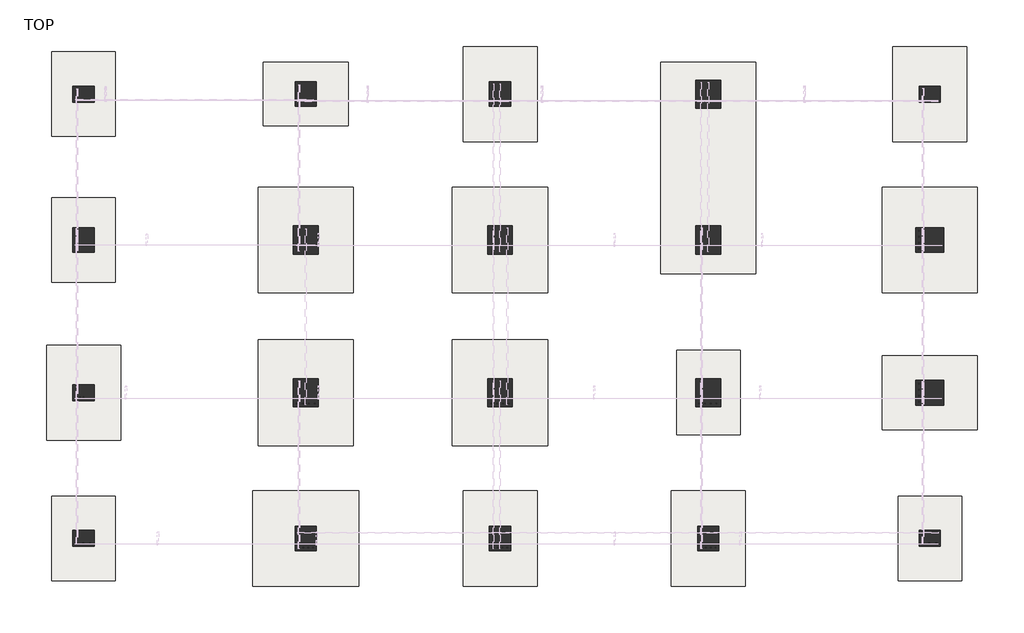
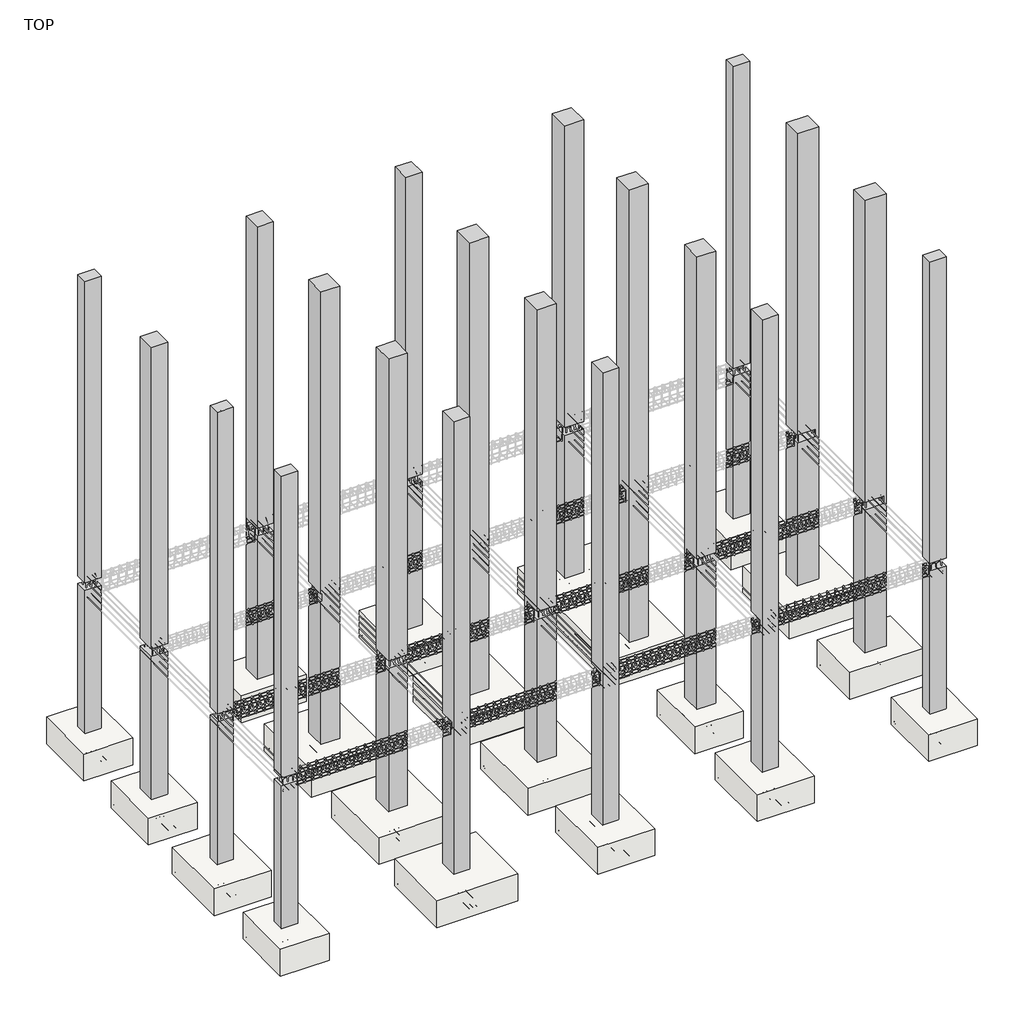
# One storey, part 1 of 8: 20 columns, 19 slabs.
"""IFC4 building model written with IfcOpenShell, lengths in millimetres."""

from ifc_helpers import new_model, si_unit, frame, origin, origin_with_axes, place, context, project, spatial, polyline, outline, extrude, faceted_brep, transform, mapped, element, save
from components import footing_rectangular_f1_21e6a39c, footing_rectangular_f2_078fe2d8, footing_rectangular_f3_af965022, footing_rectangular_f4_618a482d

model = new_model("IFC4")

# Units and contexts
model_context = context("Model", 3, world=origin())
ifc_project = project(units=[si_unit("LENGTHUNIT", "METRE", prefix="MILLI")], contexts=[model_context])

# Site, building, storey
site = spatial("IfcSite", under=ifc_project)
building = spatial("IfcBuilding", under=site)
storey = spatial("IfcBuildingStorey", under=building, Name="TOP", Elevation=0.0)

# Columns
placement = place(None, origin())
element("IfcColumn", 1, ObjectType="Concrete Rectangular : C1", at=placement, inside=storey, context=model_context, shape_type="SweptSolid", body=[
    extrude(outline(polyline([(-5012.5160601, 7636.2307576), (-5012.5160601, 7407.6307576), (-5317.3160601, 7407.6307576), (-5317.3160601, 7636.2307576), (-5012.5160601, 7636.2307576)])), origin_with_axes(), (0.0, 0.0, 1.0), 2847.6),
    extrude(outline(polyline([(-5012.5160601, 7636.2307576), (-5012.5160601, 7407.6307576), (-5317.3160601, 7407.6307576), (-5317.3160601, 7636.2307576), (-5012.5160601, 7636.2307576)])), frame((0.0, 0.0, 3000.0), z_axis=(0.0, 0.0, 1.0), x_axis=(1.0, 0.0, 0.0)), (0.0, 0.0, 1.0), 5998.464),
])
element("IfcColumn", 2, ObjectType="Concrete Rectangular : C1", at=placement, inside=storey, context=model_context, shape_type="SweptSolid", body=[
    extrude(outline(polyline([(-5012.5160601, 1235.4307576), (-5012.5160601, 1006.8307576), (-5317.3160601, 1006.8307576), (-5317.3160601, 1235.4307576), (-5012.5160601, 1235.4307576)])), origin_with_axes(), (0.0, 0.0, 1.0), 2847.6),
    extrude(outline(polyline([(-5012.5160601, 1235.4307576), (-5012.5160601, 1006.8307576), (-5317.3160601, 1006.8307576), (-5317.3160601, 1235.4307576), (-5012.5160601, 1235.4307576)])), frame((0.0, 0.0, 3000.0), z_axis=(0.0, 0.0, 1.0), x_axis=(1.0, 0.0, 0.0)), (0.0, 0.0, 1.0), 5998.464),
])
element("IfcColumn", 3, ObjectType="Concrete Rectangular : C1", at=placement, inside=storey, context=model_context, shape_type="SweptSolid", body=[
    extrude(outline(polyline([(-5012.5160601, 3335.4307576), (-5012.5160601, 3106.8307576), (-5317.3160601, 3106.8307576), (-5317.3160601, 3335.4307576), (-5012.5160601, 3335.4307576)])), origin_with_axes(), (0.0, 0.0, 1.0), 2847.6),
    extrude(outline(polyline([(-5012.5160601, 3335.4307576), (-5012.5160601, 3106.8307576), (-5317.3160601, 3106.8307576), (-5317.3160601, 3335.4307576), (-5012.5160601, 3335.4307576)])), frame((0.0, 0.0, 3000.0), z_axis=(0.0, 0.0, 1.0), x_axis=(1.0, 0.0, 0.0)), (0.0, 0.0, 1.0), 5998.464),
])
element("IfcColumn", 4, ObjectType="Concrete Rectangular : C1", at=placement, inside=storey, context=model_context, shape_type="SweptSolid", body=[
    extrude(outline(polyline([(7179.4839399, 1235.4307576), (7179.4839399, 1006.8307576), (6874.6839399, 1006.8307576), (6874.6839399, 1235.4307576), (7179.4839399, 1235.4307576)])), origin_with_axes(), (0.0, 0.0, 1.0), 2847.6),
    extrude(outline(polyline([(7179.4839399, 1235.4307576), (7179.4839399, 1006.8307576), (6874.6839399, 1006.8307576), (6874.6839399, 1235.4307576), (7179.4839399, 1235.4307576)])), frame((0.0, 0.0, 3000.0), z_axis=(0.0, 0.0, 1.0), x_axis=(1.0, 0.0, 0.0)), (0.0, 0.0, 1.0), 5998.464),
])
element("IfcColumn", 5, ObjectType="Concrete Rectangular : C1", at=placement, inside=storey, context=model_context, shape_type="SweptSolid", body=[
    extrude(outline(polyline([(7179.4839399, 7636.2307576), (7179.4839399, 7407.6307576), (6874.6839399, 7407.6307576), (6874.6839399, 7636.2307576), (7179.4839399, 7636.2307576)])), origin_with_axes(), (0.0, 0.0, 1.0), 2847.6),
    extrude(outline(polyline([(7179.4839399, 7636.2307576), (7179.4839399, 7407.6307576), (6874.6839399, 7407.6307576), (6874.6839399, 7636.2307576), (7179.4839399, 7636.2307576)])), frame((0.0, 0.0, 3000.0), z_axis=(0.0, 0.0, 1.0), x_axis=(1.0, 0.0, 0.0)), (0.0, 0.0, 1.0), 5998.464),
])
element("IfcColumn", 6, ObjectType="Concrete Rectangular : C2", at=placement, inside=storey, context=model_context, shape_type="SweptSolid", body=[
    extrude(outline(polyline([(3424.2799576, 0.0), (3017.9815576, 0.0), (3017.9815576, 2847.6), (3348.0799576, 2847.6), (3348.0799576, 3000.0), (3017.9815576, 3000.0), (3017.9815576, 8998.464), (3424.2799576, 8998.464), (3424.2799576, 0.0)])), frame((3657.2331399, 0.0, 0.0), z_axis=(1.0, 0.0, 0.0), x_axis=(0.0, 1.0, 0.0)), (0.0, 0.0, 1.0), 355.7016),
])
element("IfcColumn", 7, ObjectType="Concrete Rectangular : C2", at=placement, inside=storey, context=model_context, shape_type="Brep", body=[
    faceted_brep([(-1787.0652601, 5625.0799576, 0.0), (-1787.0652601, 5218.7815576, 0.0), (-2142.7668601, 5218.7815576, 0.0), (-2142.7668601, 5625.0799576, 0.0), (-1787.0652601, 5625.0799576, 2847.6), (-1787.0652601, 5548.8799576, 2847.6), (-1787.0652601, 5548.8799576, 3000.0), (-1787.0652601, 5625.0799576, 3000.0), (-1787.0652601, 5625.0799576, 8998.464), (-1787.0652601, 5218.7815576, 8998.464), (-2142.7668601, 5218.7815576, 8998.464), (-2142.7668601, 5218.7815576, 3000.0), (-2117.3160601, 5218.7815576, 3000.0), (-2117.3160601, 5218.7815576, 2847.6), (-2142.7668601, 5218.7815576, 2847.6), (-2142.7668601, 5625.0799576, 8998.464), (-2142.7668601, 5625.0799576, 3000.0), (-2117.3160601, 5548.8799576, 2847.6), (-2142.7668601, 5625.0799576, 2847.6), (-2117.3160601, 5548.8799576, 3000.0)], [[[0, 1, 2, 3]], [[1, 0, 4, 5, 6, 7, 8, 9]], [[2, 1, 9, 10, 11, 12, 13, 14]], [[10, 15, 16, 11]], [[15, 8, 7, 16]], [[9, 8, 15, 10]], [[14, 13, 17, 5, 4, 18]], [[12, 11, 16, 7, 6, 19]], [[13, 12, 19, 17]], [[3, 2, 14, 18]], [[5, 17, 19, 6]], [[0, 3, 18, 4]]]),
])
element("IfcColumn", 8, ObjectType="Concrete Rectangular : C2", at=placement, inside=storey, context=model_context, shape_type="SweptSolid", body=[
    extrude(outline(polyline([(5625.0799576, 0.0), (5218.7815576, 0.0), (5218.7815576, 8998.464), (5625.0799576, 8998.464), (5625.0799576, 3000.0), (5548.8799576, 3000.0), (5548.8799576, 2847.6), (5625.0799576, 2847.6), (5625.0799576, 0.0)])), frame((657.2331399, 0.0, 0.0), z_axis=(1.0, 0.0, 0.0), x_axis=(0.0, 1.0, 0.0)), (0.0, 0.0, 1.0), 355.7016),
])
element("IfcColumn", 9, ObjectType="Concrete Rectangular : C2", at=placement, inside=storey, context=model_context, shape_type="SweptSolid", body=[
    extrude(outline(polyline([(3424.2799576, 0.0), (3017.9815576, 0.0), (3017.9815576, 2847.6), (3348.0799576, 2847.6), (3348.0799576, 3000.0), (3017.9815576, 3000.0), (3017.9815576, 8998.464), (3424.2799576, 8998.464), (3424.2799576, 0.0)])), frame((657.2331399, 0.0, 0.0), z_axis=(1.0, 0.0, 0.0), x_axis=(0.0, 1.0, 0.0)), (0.0, 0.0, 1.0), 355.7016),
])
element("IfcColumn", 10, ObjectType="Concrete Rectangular : C2", at=placement, inside=storey, context=model_context, shape_type="Brep", body=[
    faceted_brep([(-1787.0652601, 3424.2799576, 0.0), (-1787.0652601, 3017.9815576, 0.0), (-2142.7668601, 3017.9815576, 0.0), (-2142.7668601, 3424.2799576, 0.0), (-1787.0652601, 3424.2799576, 8998.464), (-1787.0652601, 3017.9815576, 8998.464), (-1787.0652601, 3017.9815576, 3000.0), (-1787.0652601, 3348.0799576, 3000.0), (-1787.0652601, 3348.0799576, 2847.6), (-1787.0652601, 3017.9815576, 2847.6), (-2142.7668601, 3017.9815576, 8998.464), (-2142.7668601, 3017.9815576, 3000.0), (-2142.7668601, 3424.2799576, 8998.464), (-2142.7668601, 3424.2799576, 3000.0), (-2142.7668601, 3424.2799576, 2847.6), (-2117.3160601, 3424.2799576, 2847.6), (-2117.3160601, 3424.2799576, 3000.0), (-2117.3160601, 3348.0799576, 2847.6), (-2142.7668601, 3017.9815576, 2847.6), (-2117.3160601, 3348.0799576, 3000.0)], [[[0, 1, 2, 3]], [[1, 0, 4, 5, 6, 7, 8, 9]], [[5, 10, 11, 6]], [[10, 12, 13, 11]], [[0, 3, 14, 15, 16, 13, 12, 4]], [[5, 4, 12, 10]], [[9, 8, 17, 15, 14, 18]], [[11, 13, 16, 19, 7, 6]], [[16, 15, 17, 19]], [[3, 2, 18, 14]], [[17, 8, 7, 19]], [[2, 1, 9, 18]]]),
])
element("IfcColumn", 11, ObjectType="Concrete Rectangular : C2", at=placement, inside=storey, context=model_context, shape_type="SweptSolid", body=[
    extrude(outline(polyline([(5625.0799576, 0.0), (5218.7815576, 0.0), (5218.7815576, 8998.464), (5625.0799576, 8998.464), (5625.0799576, 3000.0), (5548.8799576, 3000.0), (5548.8799576, 2847.6), (5625.0799576, 2847.6), (5625.0799576, 0.0)])), frame((3657.2331399, 0.0, 0.0), z_axis=(1.0, 0.0, 0.0), x_axis=(0.0, 1.0, 0.0)), (0.0, 0.0, 1.0), 355.7016),
])
element("IfcColumn", 12, ObjectType="Concrete Rectangular : C2", at=placement, inside=storey, context=model_context, shape_type="SweptSolid", body=[
    extrude(outline(polyline([(7725.0799576, 0.0), (7318.7815576, 0.0), (7318.7815576, 2847.6), (7674.3307576, 2847.6), (7674.3307576, 3000.0), (7318.7815576, 3000.0), (7318.7815576, 8998.464), (7725.0799576, 8998.464), (7725.0799576, 0.0)])), frame((3657.2331399, 0.0, 0.0), z_axis=(1.0, 0.0, 0.0), x_axis=(0.0, 1.0, 0.0)), (0.0, 0.0, 1.0), 355.7016),
])
element("IfcColumn", 13, ObjectType="Concrete Rectangular : C2", at=placement, inside=storey, context=model_context, shape_type="SweptSolid", body=[
    extrude(outline(polyline([(0.0, 6823.9347399), (0.0, 7230.2331399), (8998.464, 7230.2331399), (8998.464, 6823.9347399), (3000.0, 6823.9347399), (3000.0, 7179.4839399), (2847.6, 7179.4839399), (2847.6, 6823.9347399), (0.0, 6823.9347399)])), frame((0.0, 3043.2799576, 0.0), z_axis=(0.0, 1.0, 0.0), x_axis=(0.0, 0.0, 1.0)), (0.0, 0.0, 1.0), 355.7016),
])
element("IfcColumn", 14, ObjectType="Concrete Rectangular : C2", at=placement, inside=storey, context=model_context, shape_type="SweptSolid", body=[
    extrude(outline(polyline([(0.0, 6823.9347399), (0.0, 7230.2331399), (8998.464, 7230.2331399), (8998.464, 6823.9347399), (3000.0, 6823.9347399), (3000.0, 7179.4839399), (2847.6, 7179.4839399), (2847.6, 6823.9347399), (0.0, 6823.9347399)])), frame((0.0, 5244.0799576, 0.0), z_axis=(0.0, 1.0, 0.0), x_axis=(0.0, 0.0, 1.0)), (0.0, 0.0, 1.0), 355.7016),
])
element("IfcColumn", 15, ObjectType="Concrete Rectangular : C3", at=placement, inside=storey, context=model_context, shape_type="SweptSolid", body=[
    extrude(outline(polyline([(7699.7815576, 0.0), (7344.0799576, 0.0), (7344.0799576, 2847.6), (7674.3307576, 2847.6), (7674.3307576, 3000.0), (7344.0799576, 3000.0), (7344.0799576, 8998.464), (7699.7815576, 8998.464), (7699.7815576, 0.0)])), frame((-2117.3160601, 0.0, 0.0), z_axis=(1.0, 0.0, 0.0), x_axis=(0.0, 1.0, 0.0)), (0.0, 0.0, 1.0), 304.8),
])
element("IfcColumn", 16, ObjectType="Concrete Rectangular : C3", at=placement, inside=storey, context=model_context, shape_type="SweptSolid", body=[
    extrude(outline(polyline([(-5012.5160601, 5599.7815576), (-5012.5160601, 5244.0799576), (-5317.3160601, 5244.0799576), (-5317.3160601, 5599.7815576), (-5012.5160601, 5599.7815576)])), origin_with_axes(), (0.0, 0.0, 1.0), 2847.6),
    extrude(outline(polyline([(-5012.5160601, 5599.7815576), (-5012.5160601, 5244.0799576), (-5317.3160601, 5244.0799576), (-5317.3160601, 5599.7815576), (-5012.5160601, 5599.7815576)])), frame((0.0, 0.0, 3000.0), z_axis=(0.0, 0.0, 1.0), x_axis=(1.0, 0.0, 0.0)), (0.0, 0.0, 1.0), 5998.464),
])
element("IfcColumn", 17, ObjectType="Concrete Rectangular : C3", at=placement, inside=storey, context=model_context, shape_type="SweptSolid", body=[
    extrude(outline(polyline([(1298.9815576, 0.0), (943.2799576, 0.0), (943.2799576, 8998.464), (1298.9815576, 8998.464), (1298.9815576, 3000.0), (994.1815576, 3000.0), (994.1815576, 2847.6), (1298.9815576, 2847.6), (1298.9815576, 0.0)])), frame((-2117.3160601, 0.0, 0.0), z_axis=(1.0, 0.0, 0.0), x_axis=(0.0, 1.0, 0.0)), (0.0, 0.0, 1.0), 304.8),
])
element("IfcColumn", 18, ObjectType="Concrete Rectangular : C3", at=placement, inside=storey, context=model_context, shape_type="SweptSolid", body=[
    extrude(outline(polyline([(1298.9815576, 0.0), (943.2799576, 0.0), (943.2799576, 8998.464), (1298.9815576, 8998.464), (1298.9815576, 3000.0), (994.1815576, 3000.0), (994.1815576, 2847.6), (1298.9815576, 2847.6), (1298.9815576, 0.0)])), frame((682.6839399, 0.0, 0.0), z_axis=(1.0, 0.0, 0.0), x_axis=(0.0, 1.0, 0.0)), (0.0, 0.0, 1.0), 304.8),
])
element("IfcColumn", 19, ObjectType="Concrete Rectangular : C3", at=placement, inside=storey, context=model_context, shape_type="SweptSolid", body=[
    extrude(outline(polyline([(7699.7815576, 0.0), (7344.0799576, 0.0), (7344.0799576, 2847.6), (7674.3307576, 2847.6), (7674.3307576, 3000.0), (7344.0799576, 3000.0), (7344.0799576, 8998.464), (7699.7815576, 8998.464), (7699.7815576, 0.0)])), frame((682.6839399, 0.0, 0.0), z_axis=(1.0, 0.0, 0.0), x_axis=(0.0, 1.0, 0.0)), (0.0, 0.0, 1.0), 304.8),
])
element("IfcColumn", 20, ObjectType="Concrete Rectangular : C3", at=placement, inside=storey, context=model_context, shape_type="SweptSolid", body=[
    extrude(outline(polyline([(1298.9815576, 0.0), (943.2799576, 0.0), (943.2799576, 8998.464), (1298.9815576, 8998.464), (1298.9815576, 3000.0), (994.1815576, 3000.0), (994.1815576, 2847.6), (1298.9815576, 2847.6), (1298.9815576, 0.0)])), frame((3682.6839399, 0.0, 0.0), z_axis=(1.0, 0.0, 0.0), x_axis=(0.0, 1.0, 0.0)), (0.0, 0.0, 1.0), 304.8),
])

# Slabs
footing_rectangular_f1_shape = footing_rectangular_f1_21e6a39c(model_context)
element("IfcSlab", 21, ObjectType="Footing-Rectangular : F1", at=placement, inside=storey, context=model_context, shape_type="MappedRepresentation", body=[
    mapped(footing_rectangular_f1_shape, transform((-5164.9160601, 7521.9307576, 0.0), x_axis=(1.0, 0.0, 0.0), y_axis=(0.0, 1.0, 0.0), z_axis=(0.0, 0.0, 1.0))),
])
element("IfcSlab", 22, ObjectType="Footing-Rectangular : F1", at=placement, inside=storey, context=model_context, shape_type="MappedRepresentation", body=[
    mapped(footing_rectangular_f1_shape, transform((-5164.9160601, 1121.1307576, 0.0), x_axis=(1.0, 0.0, 0.0), y_axis=(0.0, 1.0, 0.0), z_axis=(0.0, 0.0, 1.0))),
])
element("IfcSlab", 23, ObjectType="Footing-Rectangular : F1", at=placement, inside=storey, context=model_context, shape_type="MappedRepresentation", body=[
    mapped(footing_rectangular_f1_shape, transform((7027.0839399, 1121.1307576, 0.0), x_axis=(1.0, 0.0, 0.0), y_axis=(0.0, 1.0, 0.0), z_axis=(0.0, 0.0, 1.0))),
])
element("IfcSlab", 24, ObjectType="Footing-Rectangular : F1", at=placement, inside=storey, context=model_context, shape_type="MappedRepresentation", body=[
    mapped(footing_rectangular_f1_shape, transform((-5164.9160601, 5421.9307576, 0.0), x_axis=(1.0, 0.0, 0.0), y_axis=(0.0, 1.0, 0.0), z_axis=(0.0, 0.0, 1.0))),
])
element("IfcSlab", 25, ObjectType="Footing-Rectangular : F1", at=placement, inside=storey, context=model_context, shape_type="MappedRepresentation", body=[
    mapped(footing_rectangular_f1_shape, transform((-1964.9160601, 7521.9307576, 0.0), x_axis=(0.0, 1.0, 0.0), y_axis=(-1.0, 0.0, 0.0), z_axis=(0.0, 0.0, 1.0))),
])
element("IfcSlab", 26, ObjectType="Footing-Rectangular : F1", at=placement, inside=storey, context=model_context, shape_type="MappedRepresentation", body=[
    mapped(footing_rectangular_f1_shape, transform((3835.0839399, 3221.1307576, 0.0), x_axis=(-1.0, 0.0, 0.0), y_axis=(0.0, -1.0, 0.0), z_axis=(0.0, 0.0, 1.0))),
])
footing_rectangular_f2_shape = footing_rectangular_f2_078fe2d8(model_context)
element("IfcSlab", 27, ObjectType="Footing-Rectangular : F2", at=placement, inside=storey, context=model_context, shape_type="MappedRepresentation", body=[
    mapped(footing_rectangular_f2_shape, transform((-1964.9160601, 5421.9307576, 0.0), x_axis=(1.0, 0.0, 0.0), y_axis=(0.0, 1.0, 0.0), z_axis=(0.0, 0.0, 1.0))),
])
element("IfcSlab", 28, ObjectType="Footing-Rectangular : F2", at=placement, inside=storey, context=model_context, shape_type="MappedRepresentation", body=[
    mapped(footing_rectangular_f2_shape, transform((835.0839399, 3221.1307576, 0.0), x_axis=(1.0, 0.0, 0.0), y_axis=(0.0, 1.0, 0.0), z_axis=(0.0, 0.0, 1.0))),
])
element("IfcSlab", 29, ObjectType="Footing-Rectangular : F2", at=placement, inside=storey, context=model_context, shape_type="MappedRepresentation", body=[
    mapped(footing_rectangular_f2_shape, transform((835.0839399, 5421.9307576, 0.0), x_axis=(1.0, 0.0, 0.0), y_axis=(0.0, 1.0, 0.0), z_axis=(0.0, 0.0, 1.0))),
])
element("IfcSlab", 30, ObjectType="Footing-Rectangular : F2", at=placement, inside=storey, context=model_context, shape_type="MappedRepresentation", body=[
    mapped(footing_rectangular_f2_shape, transform((-1964.9160601, 3221.1307576, 0.0), x_axis=(1.0, 0.0, 0.0), y_axis=(0.0, 1.0, 0.0), z_axis=(0.0, 0.0, 1.0))),
])
element("IfcSlab", 31, ObjectType="Footing-Rectangular : F2", at=placement, inside=storey, context=model_context, shape_type="MappedRepresentation", body=[
    mapped(footing_rectangular_f2_shape, transform((7027.0839399, 5421.9307576, 0.0), x_axis=(1.0, 0.0, 0.0), y_axis=(0.0, 1.0, 0.0), z_axis=(0.0, 0.0, 1.0))),
])
element("IfcSlab", 32, ObjectType="Footing-Rectangular : F2", at=placement, inside=storey, context=model_context, shape_type="MappedRepresentation", body=[
    mapped(footing_rectangular_f2_shape, transform((-1964.9160601, 1121.1307576, 0.0), x_axis=(0.0, 1.0, 0.0), y_axis=(-1.0, 0.0, 0.0), z_axis=(0.0, 0.0, 1.0))),
])
footing_rectangular_f3_shape = footing_rectangular_f3_af965022(model_context)
element("IfcSlab", 33, ObjectType="Footing-Rectangular : F3", at=placement, inside=storey, context=model_context, shape_type="MappedRepresentation", body=[
    mapped(footing_rectangular_f3_shape, transform((835.0839399, 7521.9307576, 0.0), x_axis=(1.0, 0.0, 0.0), y_axis=(0.0, 1.0, 0.0), z_axis=(0.0, 0.0, 1.0))),
])
element("IfcSlab", 34, ObjectType="Footing-Rectangular : F3", at=placement, inside=storey, context=model_context, shape_type="MappedRepresentation", body=[
    mapped(footing_rectangular_f3_shape, transform((7027.0839399, 7521.9307576, 0.0), x_axis=(1.0, 0.0, 0.0), y_axis=(0.0, 1.0, 0.0), z_axis=(0.0, 0.0, 1.0))),
])
element("IfcSlab", 35, ObjectType="Footing-Rectangular : F3", at=placement, inside=storey, context=model_context, shape_type="MappedRepresentation", body=[
    mapped(footing_rectangular_f3_shape, transform((835.0839399, 1121.1307576, 0.0), x_axis=(1.0, 0.0, 0.0), y_axis=(0.0, 1.0, 0.0), z_axis=(0.0, 0.0, 1.0))),
])
element("IfcSlab", 36, ObjectType="Footing-Rectangular : F3", at=placement, inside=storey, context=model_context, shape_type="MappedRepresentation", body=[
    mapped(footing_rectangular_f3_shape, transform((-5164.9160601, 3221.1307576, 0.0), x_axis=(1.0, 0.0, 0.0), y_axis=(0.0, 1.0, 0.0), z_axis=(0.0, 0.0, 1.0))),
])
element("IfcSlab", 37, ObjectType="Footing-Rectangular : F3", at=placement, inside=storey, context=model_context, shape_type="MappedRepresentation", body=[
    mapped(footing_rectangular_f3_shape, transform((3835.0839399, 1121.1307576, 0.0), x_axis=(1.0, 0.0, 0.0), y_axis=(0.0, 1.0, 0.0), z_axis=(0.0, 0.0, 1.0))),
])
element("IfcSlab", 38, ObjectType="Footing-Rectangular : F3", at=placement, inside=storey, context=model_context, shape_type="MappedRepresentation", body=[
    mapped(footing_rectangular_f3_shape, transform((7027.0839399, 3221.1307576, 0.0), x_axis=(0.0, 1.0, 0.0), y_axis=(-1.0, 0.0, 0.0), z_axis=(0.0, 0.0, 1.0))),
])
footing_rectangular_f4_shape = footing_rectangular_f4_618a482d(model_context)
element("IfcSlab", 39, ObjectType="Footing-Rectangular : F4", at=placement, inside=storey, context=model_context, shape_type="MappedRepresentation", body=[
    mapped(footing_rectangular_f4_shape, transform((3835.0839399, 6455.1307576, 0.0), x_axis=(0.0, 1.0, 0.0), y_axis=(-1.0, 0.0, 0.0), z_axis=(0.0, 0.0, 1.0))),
])

save(model, "model.ifc")

# Revit data of these elements
# Grids (mm)
#   "1": line (9751.029, 7521.931) -> (-8926.836, 7521.931)
#   "4": line (9751.029, 1121.131) -> (-8926.836, 1121.131)
#   "A": line (-5164.916, 12007.297) -> (-5164.916, -940.623)
#   "C": line (835.084, 12007.297) -> (835.084, -940.623)
#   "E": line (7027.084, 12007.297) -> (7027.084, -940.623)
#   "B": line (-1964.916, 12007.297) -> (-1964.916, -940.623)
#   "D": line (3835.084, 12007.297) -> (3835.084, -940.623)
#   "2": line (9751.029, 5421.931) -> (-8926.836, 5421.931)
#   "3": line (9751.029, 3221.131) -> (-8926.836, 3221.131)
# Type "Concrete Rectangular : C1"
#   Keynote = "E"
#   b = 304.8 mm
#   h = 228.6 mm
#   Structural Material [instance default] = Concrete - Cast-in-Place Concrete
# Type "Concrete Rectangular : C2"
#   Keynote = "E"
#   b = 355.702 mm
#   h = 406.298 mm
#   Structural Material [instance default] = Concrete - Cast-in-Place Concrete
# Type "Concrete Rectangular : C3"
#   Keynote = "E"
#   b = 304.8 mm
#   h = 355.702 mm
#   Structural Material [instance default] = Concrete - Cast-in-Place Concrete
# Type "Footing-Rectangular : F1"
#   Width = 914.4 mm
#   Length = 1219.2 mm
#   Foundation Thickness = 533.4 mm
#   Structural Material [instance default] = Concrete - Cast-in-Place Concrete
#   Assembly Code = ""
# Type "Footing-Rectangular : F2"
#   Width = 1371.6 mm
#   Length = 1524 mm
#   Foundation Thickness = 533.4 mm
#   Structural Material [instance default] = Concrete - Cast-in-Place Concrete
#   Assembly Code = ""
# Type "Footing-Rectangular : F3"
#   Width = 1066.8 mm
#   Length = 1371.6 mm
#   Foundation Thickness = 533.4 mm
#   Structural Material [instance default] = Concrete - Cast-in-Place Concrete
#   Assembly Code = ""
# Type "Footing-Rectangular : F4"
#   Width = 3048 mm
#   Length = 1371.6 mm
#   Foundation Thickness = 533.4 mm
#   Structural Material [instance default] = Concrete - Cast-in-Place Concrete
#   Assembly Code = ""
# Elements 1, 2, 3, 4, 5 (IfcColumn, "Concrete Rectangular : C1")
#   Structural Material = Concrete - Cast-in-Place Concrete
#   Phase Created = New Construction
#   Materials on its faces: "Concrete - Cast-in-Place Concrete"
# Elements 6, 7, 8, 9, 10, 11, 12, 13, 14 (IfcColumn, "Concrete Rectangular : C2")
#   Structural Material = Concrete - Cast-in-Place Concrete
#   Phase Created = New Construction
#   Materials on its faces: "Concrete - Cast-in-Place Concrete"
# Elements 15, 16, 17, 18, 19, 20 (IfcColumn, "Concrete Rectangular : C3")
#   Structural Material = Concrete - Cast-in-Place Concrete
#   Phase Created = New Construction
#   Materials on its faces: "Concrete - Cast-in-Place Concrete"
# Elements 21, 22, 23, 24, 25, 26 (IfcSlab, "Footing-Rectangular : F1")
#   Structural Material = Concrete - Cast-in-Place Concrete
#   Phase Created = New Construction
#   Materials on its faces: "Concrete - Cast-in-Place Concrete"
# Elements 27, 28, 29, 30, 31, 32 (IfcSlab, "Footing-Rectangular : F2")
#   Structural Material = Concrete - Cast-in-Place Concrete
#   Phase Created = New Construction
#   Materials on its faces: "Concrete - Cast-in-Place Concrete"
# Elements 33, 34, 35, 36, 37, 38 (IfcSlab, "Footing-Rectangular : F3")
#   Structural Material = Concrete - Cast-in-Place Concrete
#   Phase Created = New Construction
#   Materials on its faces: "Concrete - Cast-in-Place Concrete"
# Element 39 (IfcSlab, "Footing-Rectangular : F4")
#   Structural Material = Concrete - Cast-in-Place Concrete
#   Phase Created = New Construction
#   Materials on its faces: "Concrete - Cast-in-Place Concrete"
# Materials
#   "Concrete - Cast-in-Place Concrete": class "Concrete", colour RGB 192 192 192, transparency 0, Cost = 0
